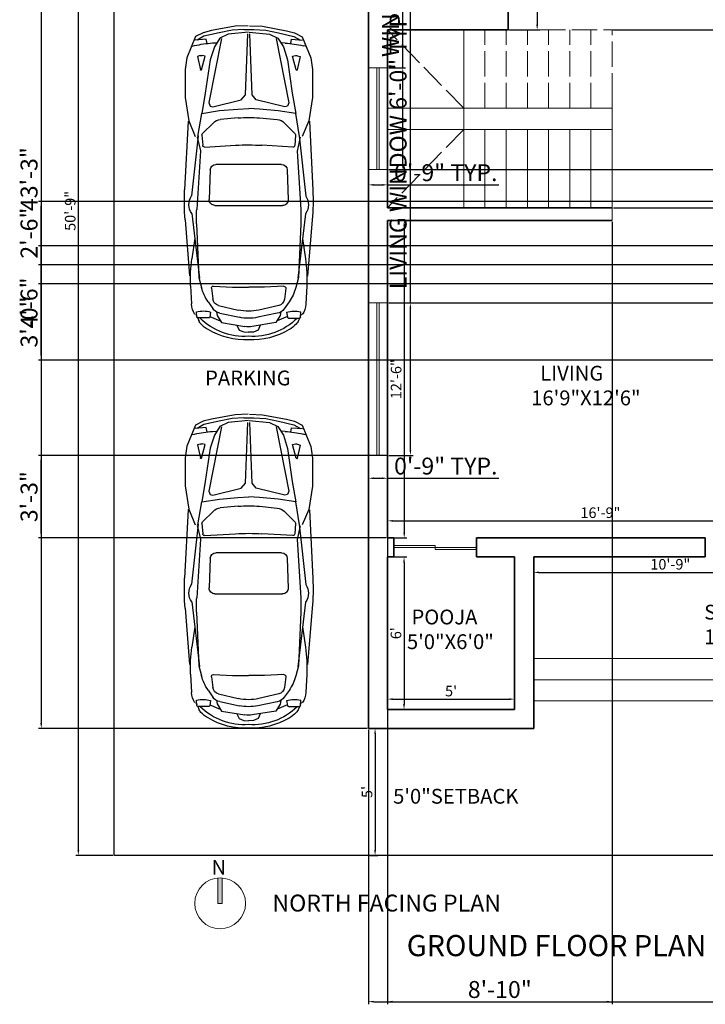
# Model space of a CAD drawing. Units: inches. Extents: x 3394 to 4794, y 965 to 1718.
# Tile 12 of 15: x 4177 to 4500, y 987 to 1453. Entities that reach past the tile are written whole.
import ezdxf

# ---------------------------------------------------------------- set-up
doc = ezdxf.new("R2010")
doc.units = ezdxf.units.IN
doc.linetypes.add('ACAD_ISO02W100', pattern=[15, 12, -3])
for name, color, linetype, lineweight in [('A-ANNO-DIMS', 2, 'Continuous', 13), ('A-ANNO-SYMB', 7, 'Continuous', 18), ('A-ANNO-TEXT', 7, 'Continuous', 18), ('A-ANNO-TITL', 7, 'Continuous', 25), ('A-AREA-IDEN', 7, 'Continuous', 18), ('A-DOOR', 4, 'Continuous', 18), ('A-FLOR-STRS', 7, 'Continuous', 18), ('A-FLOR-STRS-OVHD', 7, 'ACAD_ISO02W100', 13), ('A-GLAZ', 4, 'Continuous', 18), ('A-WALL', 7, 'Continuous', 35), ('C-PRKG-VEHI', 8, 'Continuous', 13), ('C-PROP', 7, 'Continuous', 25)]:
    doc.layers.add(name, color=color, linetype=linetype, lineweight=lineweight)
doc.layers.add('L9012X$0', color=2, linetype='Continuous')
doc.styles.get("Standard").update_dxf_attribs({"font": 'arial.ttf'})
doc.dimstyles.new('ISO-25', dxfattribs={"dimtxt": 8, "dimasz": 2.5, "dimexe": 1.25, "dimexo": 0.625, "dimtad": 1, "dimlunit": 3, "dimtxsty": 'Standard', "dimcen": 2.5, "dimadec": 0, "dimazin": 0, "dimtfac": 1, "dimtmove": 0, "dimatfit": 3, "dimfxl": 1, "dimarcsym": 0})

# ---------------------------------------------------------------- blocks, each defined once
blk = doc.blocks.new('A1099DC')
at = {"color": 0, "linetype": 'ByBlock'}
for p, q in [((1279.298465, 804.448389), (2201.430588, 851.890505)), ((2602.736326, 846.078152), (3356.693814, 785.353187)), ((139.051458, 595.027331), (190.951238, 683.213377)), ((179.200345, 564.515703), (190.951238, 709.631982)), ((272.228253, 749.073842), (265.114727, 718.465169)), ((398.733388, 644.315148), (411.280494, 678.748261)), ((411.280494, 678.748261), (588.616917, 641.417897)), ((1482.852352, 674.283145), (1175.286956, 622.180789)), ((1475.52921, 670.226262), (2282.402739, 758.004075)), ((1494.603245, 682.841284), (1678.210958, 641.166865)), ((1678.210958, 641.166865), (2462.684993, 690.847736)), ((2519.280414, 756.817792), (3387.476361, 653.818028)), ((2656.476214, 692.831247), (3376.704709, 662.004075)), ((2851.341839, 715.213377), (3126.60716, 755.701993)), ((3376.704709, 662.004075), (3510.708679, 626.736433)), ((3488.458929, 772.663345), (3732.658862, 759.86454)), ((3909.27561, 688.812956), (3837.725727, 693.401722)), ((3867.794139, 700.329656), (3900.059395, 686.767505)), ((3921.162781, 527.618662), (3921.162781, 676.138994)), ((3925.383812, 676.122818), (3955.306409, 663.545364)), ((92.537504, 388.14361), (139.051458, 595.027331)), ((236.043912, 551.980927), (179.200345, 564.515703)), ((405.405047, 577.538958), (396.874865, 615.894428)), ((589.014326, 626.599587), (405.405047, 577.538958)), ((1300.814287, 466.658131), (1445.712032, 613.104998)), ((1465.665584, 620.56924), (1602.893878, 610.287296)), ((1626.354615, 583.507504), (1602.652901, 169.222264)), ((3704.596898, 536.993674), (3795.675135, 473.385795)), ((229.117398, 477.634662), (225.714299, 427.957563)), ((1860.238743, -448.635916), (1859.369151, 433.397797)), ((1933.148906, 509.557888), (2330.980062, 522.200075)), ((2409.60024, 445.938054), (2410.49349, -460.09121)), ((3493.960271, 465.734554), (3507.923021, 209.166865)), ((3522.252709, 492.345257), (3666.066199, 475.644444)), ((3753.293176, 397.789551), (3815.226005, 132.124765)), ((3839.396146, 426.841284), (3888.358202, 417.538958)), ((3841.786866, 503.451367), (3910.58243, 515.096797)), ((3888.358202, 417.538958), (3983.199613, 359.957848)), ((3901.001848, 514.780764), (3957.150905, 375.772812)), ((57.774444, 216.608726), (92.537504, 388.14361)), ((1235.045743, 136.116317), (1257.419842, 373.755108)), ((3857.610793, 379.525702), (3912.067615, 118.157673)), ((3983.199613, 359.957848), (4035.448301, 43.94997)), ((49.168662, 58.00681), (57.774444, 216.608726)), ((3507.923021, 209.166865), (3507.64153, -4.333678)), ((4019.086894, 150.376168), (4084.69605, 122.469191)), ((4084.69605, 122.469191), (4109.177079, 60.329656)), ((4109.177079, 60.329656), (4113.094043, -5.158716)), ((49.301278, -76.507426), (58.219773, -235.092064)), ((3508.347273, -221.154823), (3507.644805, -7.65525)), ((3858.370276, -390.823819), (3912.311631, -129.348921)), ((3983.920268, -371.008369), (4035.545755, -54.898082)), ((4084.948231, -133.320044), (4109.306686, -71.132359)), ((4109.306686, -71.132359), (4113.094514, -5.636391)), ((58.219773, -235.092064), (93.320996, -406.558069)), ((1235.330373, -152.586046), (1258.173002, -390.180259)), ((1627.520644, -599.204785), (1603.002095, -184.967086)), ((3494.890446, -477.749545), (3508.347273, -221.154823)), ((3754.088875, -409.293325), (3815.497749, -143.506937)), ((4019.394229, -161.356334), (4084.948231, -133.320044)), ((3889.19258, -428.776374), (3983.920268, -371.008369)), ((3902.027941, -525.993061), (3957.902795, -386.874665)), ((93.320996, -406.558069), (140.24279, -613.349673)), ((230.077082, -495.779641), (226.576036, -446.109349)), ((1301.750547, -482.997536), (1446.936772, -629.158411)), ((1934.168526, -524.650381), (2332.023837, -536.508105)), ((3523.2353, -504.304409), (3667.01558, -487.320059)), ((3705.667171, -548.593196), (3796.61981, -484.805853)), ((3840.248961, -438.175225), (3889.19258, -428.776374)), ((3842.790735, -514.780444), (3911.609128, -526.290202)), ((140.24279, -613.349673), (192.316354, -701.433212)), ((237.150178, -570.112104), (180.331436, -582.758939)), ((180.331436, -582.758939), (192.368445, -727.851766)), ((406.561378, -595.336142), (398.106841, -633.708356)), ((590.267037, -644.034637), (406.561378, -595.336142)), ((412.636377, -696.533662), (589.898847, -658.853701)), ((1484.19765, -690.263206), (1176.530118, -638.767405)), ((1466.905004, -636.583294), (1604.112757, -626.030785)), ((1495.965396, -698.798158), (1679.490579, -656.761786)), ((1679.490579, -656.761786), (2464.061049, -704.895745)), ((3378.022114, -674.249887), (3511.956283, -638.718087)), ((3922.214148, -538.79118), (3922.506998, -687.311224)), ((273.723073, -767.133288), (266.549207, -736.538701)), ((400.0214, -662.125356), (412.636377, -696.533662)), ((1476.866524, -686.22077), (2283.911563, -772.40743)), ((2520.786439, -770.754078), (3388.777604, -666.042617)), ((2657.855804, -706.497136), (3378.022114, -674.249887)), ((2852.765183, -728.494989), (3128.109803, -768.440762)), ((3489.994314, -784.688586), (3734.168535, -771.408296)), ((3910.644841, -700.0086), (3839.104145, -704.738438)), ((3869.186159, -711.60707), (3901.424611, -697.981326)), ((3926.727989, -687.286725), (3956.625729, -674.650294)), ((1280.900818, -820.829563), (2203.124693, -866.453338)), ((2604.418191, -859.849707), (3358.254477, -797.638217))]:
    blk.add_line(p, q, dxfattribs=at)
for points in [[(-0.000783, 0.794772), (5.385043, 172.701749), (63.649891, 493.818028), (92.537504, 603.957563), (144.437284, 705.166865), (428.417214, 824.236633), (585.095796, 846.190121), (961.406447, 846.190121), (1274.27399, 797.818028), (1482.852352, 709.631982)], [(83.345007, -3.206171), (111.32237, 268.957533), (164.563706, 379.583828), (279.999271, 453.709838), (456.549665, 511.628518), (901.254996, 574.918954), (1175.286956, 622.180789), (1137.52997, 385.548359), (1118.345181, 137.317882), (1109.829198, -8.358455)], [(168.178729, 359.003083), (1030.214866, 528.397865), (1077.798844, 510.531569), (1086.170082, 475.285426), (992.832238, 91.960378), (924.218938, 35.478085), (108.447994, 6.034416)], [(0.019119, -19.392451), (5.743899, -191.288474), (64.641806, -512.289243), (93.746535, -622.371603), (145.845778, -723.478374), (430.059935, -841.987962), (586.7815, -863.632471), (963.091723, -863.198028), (1275.863278, -814.209121), (1484.26735, -725.611974)], [(83.356858, -15.227176), (111.870816, -287.335185), (165.330179, -397.856284), (280.911681, -471.754535), (457.575935, -529.324983), (902.4055, -592.045995), (1176.530118, -638.767405), (1138.306616, -402.209884), (1118.632407, -154.017717), (1109.829198, -8.358455)], [(168.904615, -377.268451), (1031.273389, -545.270714), (1078.822046, -527.310627), (1087.123771, -492.048047), (993.030273, -108.907787), (924.305735, -52.560894), (108.478017, -24.418246)]]:
    blk.add_lwpolyline(points, dxfattribs=at)
for centre, radius, start, end in [((2358.037832, -2192.08357), 3048, 85.395244, 92.945173), ((2399.99649, 588.663508), 206.166238, 54.649181, 124.776949), ((1749.553982, 373.478072), 1524, 166.916578, 176.08111), ((2578.271641, -1134.295865), 1828.8, 87.549126, 93.623712), ((3392.740754, -1053.630025), 1828.8, 86.999806, 98.367602), ((3718.678317, 475.802507), 284.405862, 57.329946, 87.182375), ((4191.049821, 605.937201), 363.988953, 166.096081, 196.353514), ((3908.462781, 676.138994), 12.7, 0, 86.330429), ((3896.252417, 523.051998), 152.4, 46.38363, 67.20138), ((446.46332, 626.922805), 50.8, 159.97873, 192.538409), ((587.047263, 633.961317), 7.62, 284.960009, 78.112462), ((1463.767788, 595.240237), 25.4, 85.715073, 135.304647), ((1600.996082, 584.958293), 25.4, 356.725615, 85.715073), ((3355.555414, 37.211519), 609.6, 55.070043, 75.255062), ((3320.85101, 50.338397), 847.430844, 356.245089, 44.519453), ((3700.933354, 318.064082), 435.542335, 30.457681, 46.38363), ((3204.184594, 25.950693), 1011.814461, 358.069446, 30.457681), ((1409.148822, 359.469565), 152.4, 135.304647, 174.62136), ((1935.569151, 433.396333), 76.2, 91.82012, 179.9989), ((2333.400307, 446.03852), 76.2, 359.924458, 91.82012), ((3519.322741, 467.114813), 25.4, 83.37601, 183.115039), ((3654.346327, 374.722669), 101.6, 13.122645, 83.37601), ((3708.414764, 348.440256), 152.4, 11.769371, 55.070043), ((3908.462781, 527.618662), 12.7, 279.607718, 0), ((2752.335538, -6.739118), 1524, 174.62136, 185.491615), ((4645.676894, -4.872483), 3048, 176.725615, 183.38736), ((1266.577845, -8.050136), 1219.2, 176.894161, 183.218814), ((3221.54491, -6.276527), 609.6, 346.99033, 13.122645), ((3315.283499, -6.18411), 609.6, 348.343604, 11.769371), ((3734.73098, -5.770579), 304.8, 350.724636, 9.388339), ((3320.962449, -62.69553), 847.430844, 315.593523, 3.867886), ((3204.248172, -38.537915), 1011.814461, 329.655294, 2.043529), ((1409.873518, -375.595566), 152.4, 185.491615, 224.808328), ((3709.113243, -360.032616), 152.4, 305.042932, 348.343604), ((1750.305335, -388.625277), 1524, 184.031865, 193.196397), ((1936.438592, -448.484202), 76.2, 180.114076, 268.292856), ((2334.293902, -460.341926), 76.2, 268.292856, 0.188517), ((3520.255588, -479.079792), 25.4, 176.997936, 276.736965), ((3655.096735, -386.42159), 101.6, 276.736965, 346.99033), ((4192.255091, -616.577407), 363.988953, 163.759461, 194.016894), ((3909.514173, -538.816222), 12.7, 0.112975, 80.505257), ((447.716945, -644.638934), 50.8, 167.574566, 200.134245), ((588.314493, -651.400231), 7.62, 282.000513, 75.152966), ((1464.957267, -611.258083), 25.4, 224.808328, 274.397903), ((1602.165021, -600.705574), 25.4, 274.397903, 3.38736), ((3355.640902, -49.500248), 609.6, 284.857913, 305.042932), ((3897.294828, -534.273643), 152.4, 292.911596, 313.729345), ((3701.571953, -329.671253), 435.542335, 313.729345, 329.655294), ((2401.171182, -602.835323), 206.166238, 235.336026, 305.463794), ((2576.048678, 1120.472221), 1828.8, 266.489263, 272.563849), ((3390.675263, 1041.412497), 1828.8, 261.745373, 273.113169), ((3719.627907, -487.374382), 284.405862, 272.930601, 302.78303), ((3909.807023, -687.336265), 12.7, 273.782546, 0.112975), ((2353.729565, 2177.823616), 3048, 267.167802, 274.717731)]:
    blk.add_arc(centre, radius, start, end, dxfattribs=at)
blk = doc.blocks.new('VI')
at = {"layer": 'L9012X$0'}
blk.add_blockref('A1099DC', (0, 0), dxfattribs=at)
blk = doc.blocks.new('*D33')
at = {"layer": 'A-ANNO-DIMS', "color": 0, "lineweight": -2, "transparency": 16777216}
for p, q in [((4407.9, 1573.68), (4422.16, 1573.68)), ((4420.91, 1571.18), (4420.91, 1450.18)), ((4407.9, 1447.68), (4422.16, 1447.68))]:
    blk.add_line(p, q, dxfattribs=at)
at = {"layer": 'A-ANNO-DIMS', "color": 0, "transparency": 16777216}
for points in [[(4420.49, 1571.18), (4421.33, 1571.18), (4420.91, 1573.68)], [(4420.49, 1450.18), (4421.33, 1450.18), (4420.91, 1447.68)]]:
    blk.add_solid(points, dxfattribs=at)
at = {"layer": 'Defpoints', "color": 0, "transparency": 16777216}
for p in [(4407.27, 1573.68), (4407.27, 1447.68), (4420.91, 1447.68)]:
    blk.add_point(p, dxfattribs=at)
at = {"layer": 'A-ANNO-DIMS', "color": 0, "transparency": 16777216, "insert": (4417.73, 1510.68), "char_height": 5, "attachment_point": 5, "rotation": 90}
blk.add_mtext('10\'-6"', dxfattribs=at)
blk = doc.blocks.new('*D34')
at = {"layer": 'A-ANNO-DIMS', "color": 0, "lineweight": -2, "transparency": 16777216}
for p, q in [((4350.9, 1198.68), (4359.32, 1198.68)), ((4358.07, 1196.18), (4358.07, 1129.18)), ((4350.9, 1126.68), (4359.32, 1126.68))]:
    blk.add_line(p, q, dxfattribs=at)
at = {"layer": 'A-ANNO-DIMS', "color": 0, "transparency": 16777216}
for points in [[(4357.65, 1196.18), (4358.48, 1196.18), (4358.07, 1198.68)], [(4357.65, 1129.18), (4358.48, 1129.18), (4358.07, 1126.68)]]:
    blk.add_solid(points, dxfattribs=at)
at = {"layer": 'Defpoints', "color": 0, "transparency": 16777216}
for p in [(4350.27, 1198.68), (4350.27, 1126.68), (4358.07, 1126.68)]:
    blk.add_point(p, dxfattribs=at)
at = {"layer": 'A-ANNO-DIMS', "color": 0, "transparency": 16777216, "insert": (4354.89, 1162.68), "char_height": 5, "attachment_point": 5, "rotation": 90}
blk.add_mtext("6'", dxfattribs=at)
blk = doc.blocks.new('*D35')
at = {"layer": 'A-ANNO-DIMS', "color": 0, "lineweight": -2, "transparency": 16777216}
for p, q in [((4350.27, 1127.31), (4350.27, 1132.77)), ((4352.77, 1131.52), (4407.77, 1131.52)), ((4410.27, 1127.31), (4410.27, 1132.77))]:
    blk.add_line(p, q, dxfattribs=at)
at = {"layer": 'A-ANNO-DIMS', "color": 0, "transparency": 16777216}
for points in [[(4352.77, 1131.94), (4352.77, 1131.11), (4350.27, 1131.52)], [(4407.77, 1131.94), (4407.77, 1131.11), (4410.27, 1131.52)]]:
    blk.add_solid(points, dxfattribs=at)
at = {"layer": 'Defpoints', "color": 0, "transparency": 16777216}
for p in [(4410.27, 1131.52), (4350.27, 1126.68), (4410.27, 1126.68)]:
    blk.add_point(p, dxfattribs=at)
at = {"layer": 'A-ANNO-DIMS', "color": 0, "transparency": 16777216, "insert": (4380.27, 1134.69), "char_height": 5, "attachment_point": 5}
blk.add_mtext("5'", dxfattribs=at)
blk = doc.blocks.new('*D36')
at = {"layer": 'A-ANNO-DIMS', "color": 0, "lineweight": -2, "transparency": 16777216}
for p, q in [((4419.27, 1198.06), (4419.27, 1190.15)), ((4548.27, 1198.06), (4548.27, 1190.15)), ((4421.77, 1191.4), (4545.77, 1191.4))]:
    blk.add_line(p, q, dxfattribs=at)
at = {"layer": 'A-ANNO-DIMS', "color": 0, "transparency": 16777216}
for points in [[(4421.77, 1191.81), (4421.77, 1190.98), (4419.27, 1191.4)], [(4545.77, 1191.81), (4545.77, 1190.98), (4548.27, 1191.4)]]:
    blk.add_solid(points, dxfattribs=at)
at = {"layer": 'Defpoints', "color": 0, "transparency": 16777216}
for p in [(4419.27, 1198.68), (4548.27, 1198.68), (4548.27, 1191.4)]:
    blk.add_point(p, dxfattribs=at)
at = {"layer": 'A-ANNO-DIMS', "color": 0, "transparency": 16777216, "insert": (4483.77, 1194.58), "char_height": 5, "attachment_point": 5}
blk.add_mtext('10\'-9"', dxfattribs=at)
blk = doc.blocks.new('*D39')
at = {"layer": 'A-ANNO-DIMS', "color": 0, "lineweight": -2, "transparency": 16777216}
for p, q in [((4341.9, 1117.68), (4345.65, 1117.68)), ((4344.4, 1115.18), (4344.4, 1060.18)), ((4341.9, 1057.68), (4345.65, 1057.68))]:
    blk.add_line(p, q, dxfattribs=at)
at = {"layer": 'A-ANNO-DIMS', "color": 0, "transparency": 16777216}
for points in [[(4343.99, 1115.18), (4344.82, 1115.18), (4344.4, 1117.68)], [(4343.99, 1060.18), (4344.82, 1060.18), (4344.4, 1057.68)]]:
    blk.add_solid(points, dxfattribs=at)
at = {"layer": 'Defpoints', "color": 0, "transparency": 16777216}
for p in [(4341.27, 1117.68), (4341.27, 1057.68), (4344.4, 1057.68)]:
    blk.add_point(p, dxfattribs=at)
at = {"layer": 'A-ANNO-DIMS', "color": 0, "transparency": 16777216, "insert": (4341.24, 1087.68), "char_height": 5, "attachment_point": 5, "rotation": 90}
blk.add_mtext("5'", dxfattribs=at)
blk = doc.blocks.new('*D40')
at = {"layer": 'A-ANNO-DIMS', "color": 0, "lineweight": -2, "transparency": 16777216}
for p, q in [((4350.9, 1357.68), (4359.41, 1357.68)), ((4358.16, 1355.18), (4358.16, 1210.18)), ((4350.9, 1207.68), (4359.41, 1207.68))]:
    blk.add_line(p, q, dxfattribs=at)
at = {"layer": 'A-ANNO-DIMS', "color": 0, "transparency": 16777216}
for points in [[(4357.74, 1355.18), (4358.57, 1355.18), (4358.16, 1357.68)], [(4357.74, 1210.18), (4358.57, 1210.18), (4358.16, 1207.68)]]:
    blk.add_solid(points, dxfattribs=at)
at = {"layer": 'Defpoints', "color": 0, "transparency": 16777216}
for p in [(4350.27, 1357.68), (4350.27, 1207.68), (4358.16, 1207.68)]:
    blk.add_point(p, dxfattribs=at)
at = {"layer": 'A-ANNO-DIMS', "color": 0, "transparency": 16777216, "insert": (4354.98, 1282.68), "char_height": 5, "attachment_point": 5, "rotation": 90}
blk.add_mtext('12\'-6"', dxfattribs=at)
blk = doc.blocks.new('*D41')
at = {"layer": 'A-ANNO-DIMS', "color": 0, "lineweight": -2, "transparency": 16777216}
for p, q in [((4350.27, 1208.31), (4350.27, 1217.01)), ((4352.77, 1215.76), (4548.77, 1215.76)), ((4551.27, 1208.31), (4551.27, 1217.01))]:
    blk.add_line(p, q, dxfattribs=at)
at = {"layer": 'A-ANNO-DIMS', "color": 0, "transparency": 16777216}
for points in [[(4352.77, 1216.17), (4352.77, 1215.34), (4350.27, 1215.76)], [(4548.77, 1216.17), (4548.77, 1215.34), (4551.27, 1215.76)]]:
    blk.add_solid(points, dxfattribs=at)
at = {"layer": 'Defpoints', "color": 0, "transparency": 16777216}
for p in [(4551.27, 1215.76), (4350.27, 1207.68), (4551.27, 1207.68)]:
    blk.add_point(p, dxfattribs=at)
at = {"layer": 'A-ANNO-DIMS', "color": 0, "transparency": 16777216, "insert": (4450.77, 1218.94), "char_height": 5, "attachment_point": 5}
blk.add_mtext('16\'-9"', dxfattribs=at)
blk = doc.blocks.new('*D53')
at = {"layer": 'A-ANNO-DIMS', "color": 0, "lineweight": -2, "transparency": 16777216}
for p, q in [((4220.65, 1666.68), (4203.08, 1666.68)), ((4204.33, 1060.18), (4204.33, 1664.18)), ((4220.65, 1057.68), (4203.08, 1057.68))]:
    blk.add_line(p, q, dxfattribs=at)
at = {"layer": 'A-ANNO-DIMS', "color": 0, "transparency": 16777216}
for points in [[(4203.92, 1664.18), (4204.75, 1664.18), (4204.33, 1666.68)], [(4203.92, 1060.18), (4204.75, 1060.18), (4204.33, 1057.68)]]:
    blk.add_solid(points, dxfattribs=at)
at = {"layer": 'Defpoints', "color": 0, "transparency": 16777216}
for p in [(4204.33, 1666.68), (4221.27, 1666.68), (4221.27, 1057.68)]:
    blk.add_point(p, dxfattribs=at)
at = {"layer": 'A-ANNO-DIMS', "color": 0, "transparency": 16777216, "insert": (4201.15, 1362.18), "char_height": 5, "attachment_point": 5, "rotation": 90}
blk.add_mtext('50\'-9"', dxfattribs=at)
blk = doc.blocks.new('WIN-48IN')
for p, q in [((9, 48), (0, 48)), ((4, 0), (4, 48)), ((5, 0), (5, 48)), ((9, 0), (0, 0))]:
    blk.add_line(p, q)
blk = doc.blocks.new('WIN-72IN')
for p, q in [((9, 72), (0, 72)), ((4, 0), (4, 72)), ((5, 0), (5, 72)), ((9, 0), (0, 0))]:
    blk.add_line(p, q)
blk = doc.blocks.new('DOOR-SLIDING-39IN')
for p, q in [((0, 2), (19.5, 2)), ((0, 1), (39, 1)), ((19.5, 2), (19.5, 0)), ((19.5, 0), (39, 0))]:
    blk.add_line(p, q)
blk = doc.blocks.new('NORTH-ARROW-PLAN')
at = {"transparency": 33554687}
h = blk.add_hatch(color=256, dxfattribs=at)
h.dxf.hatch_style = 1
h.paths.add_polyline_path([(13, 12), (11, 12), (11, 23.96, -0.020861), (12, 24, -0.020861), (13, 23.96)])
for p, q in [((11, 24), (11, 12)), ((13, 12), (13, 23.96)), ((11, 12), (13, 12))]:
    blk.add_line(p, q)
blk.add_circle((12, 12), 12)
blk.add_text('N', height=6.9).set_placement((7.98, 25.6))
blk = doc.blocks.new('STAIR-SITOUT-3STEP')
for p, q in [((129, 68), (129, 20)), ((139, 68), (139, 10)), ((149, 68), (149, 0)), ((0, 20), (129, 20)), ((0, 10), (139, 10)), ((0, 0), (149, 0))]:
    blk.add_line(p, q)
blk = doc.blocks.new('*D62')
at = {"layer": 'A-ANNO-DIMS', "color": 0, "lineweight": -2, "transparency": 16777216}
for p, q in [((4357.47, 1429.68), (4357.47, 1534.67)), ((4350.9, 1429.68), (4358.72, 1429.68)), ((4357.47, 1384.18), (4357.47, 1427.18)), ((4350.9, 1381.68), (4358.72, 1381.68))]:
    blk.add_line(p, q, dxfattribs=at)
at = {"layer": 'A-ANNO-DIMS', "color": 0, "transparency": 16777216}
for points in [[(4357.05, 1427.18), (4357.89, 1427.18), (4357.47, 1429.68)], [(4357.05, 1384.18), (4357.89, 1384.18), (4357.47, 1381.68)]]:
    blk.add_solid(points, dxfattribs=at)
at = {"layer": 'Defpoints', "color": 0, "transparency": 16777216}
for p in [(4350.27, 1429.68), (4357.47, 1429.68), (4350.27, 1381.68)]:
    blk.add_point(p, dxfattribs=at)
at = {"layer": 'A-ANNO-DIMS', "color": 0, "transparency": 16777216, "insert": (4352.71, 1483.42), "char_height": 8, "attachment_point": 5, "rotation": 90}
blk.add_mtext('WINDOW 4\'-0" TYP.', dxfattribs=at)
blk = doc.blocks.new('*D63')
at = {"layer": 'A-ANNO-DIMS', "color": 0, "lineweight": -2, "transparency": 16777216}
for p, q in [((4341.27, 1381.06), (4341.27, 1373.23)), ((4350.27, 1381.06), (4350.27, 1373.23)), ((4343.77, 1374.48), (4347.77, 1374.48)), ((4350.27, 1374.48), (4402.78, 1374.48))]:
    blk.add_line(p, q, dxfattribs=at)
at = {"layer": 'A-ANNO-DIMS', "color": 0, "transparency": 16777216}
for points in [[(4343.77, 1374.9), (4343.77, 1374.07), (4341.27, 1374.48)], [(4347.77, 1374.9), (4347.77, 1374.07), (4350.27, 1374.48)]]:
    blk.add_solid(points, dxfattribs=at)
at = {"layer": 'Defpoints', "color": 0, "transparency": 16777216}
for p in [(4341.27, 1381.68), (4350.27, 1381.68), (4350.27, 1374.48)]:
    blk.add_point(p, dxfattribs=at)
at = {"layer": 'A-ANNO-DIMS', "color": 0, "transparency": 16777216, "insert": (4377.78, 1379.19), "char_height": 8, "attachment_point": 5}
blk.add_mtext('0\'-9" TYP.', dxfattribs=at)
blk = doc.blocks.new('*D66')
at = {"layer": 'A-ANNO-DIMS', "color": 0, "lineweight": -2, "transparency": 16777216}
for p, q in [((4361.07, 1318.68), (4361.07, 1462.73)), ((4350.9, 1318.68), (4362.32, 1318.68)), ((4361.07, 1249.18), (4361.07, 1316.18)), ((4350.9, 1246.68), (4362.32, 1246.68))]:
    blk.add_line(p, q, dxfattribs=at)
at = {"layer": 'A-ANNO-DIMS', "color": 0, "transparency": 16777216}
for points in [[(4360.65, 1316.18), (4361.49, 1316.18), (4361.07, 1318.68)], [(4360.65, 1249.18), (4361.49, 1249.18), (4361.07, 1246.68)]]:
    blk.add_solid(points, dxfattribs=at)
at = {"layer": 'Defpoints', "color": 0, "transparency": 16777216}
for p in [(4350.27, 1318.68), (4361.07, 1318.68), (4350.27, 1246.68)]:
    blk.add_point(p, dxfattribs=at)
at = {"layer": 'A-ANNO-DIMS', "color": 0, "transparency": 16777216, "insert": (4356.31, 1391.96), "char_height": 8, "attachment_point": 5, "rotation": 90}
blk.add_mtext('LIVING WINDOW 6\'-0" TYP.', dxfattribs=at)
blk = doc.blocks.new('*D67')
at = {"layer": 'A-ANNO-DIMS', "color": 0, "lineweight": -2, "transparency": 16777216}
for p, q in [((4341.27, 1246.06), (4341.27, 1234.63)), ((4350.27, 1246.06), (4350.27, 1234.63)), ((4343.77, 1235.88), (4347.77, 1235.88)), ((4350.27, 1235.88), (4402.78, 1235.88))]:
    blk.add_line(p, q, dxfattribs=at)
at = {"layer": 'A-ANNO-DIMS', "color": 0, "transparency": 16777216}
for points in [[(4343.77, 1236.3), (4343.77, 1235.47), (4341.27, 1235.88)], [(4347.77, 1236.3), (4347.77, 1235.47), (4350.27, 1235.88)]]:
    blk.add_solid(points, dxfattribs=at)
at = {"layer": 'Defpoints', "color": 0, "transparency": 16777216}
for p in [(4341.27, 1246.68), (4350.27, 1246.68), (4350.27, 1235.88)]:
    blk.add_point(p, dxfattribs=at)
at = {"layer": 'A-ANNO-DIMS', "color": 0, "transparency": 16777216, "insert": (4377.78, 1240.59), "char_height": 8, "attachment_point": 5}
blk.add_mtext('0\'-9" TYP.', dxfattribs=at)
blk = doc.blocks.new('*D106')
at = {"layer": 'A-ANNO-DIMS', "color": 0, "lineweight": -2, "transparency": 16777216}
for p, q in [((4704.27, 1198.06), (4704.27, 987.36)), ((4341.27, 1117.06), (4341.27, 987.36)), ((4343.77, 988.61), (4701.77, 988.61))]:
    blk.add_line(p, q, dxfattribs=at)
at = {"layer": 'A-ANNO-DIMS', "color": 0, "transparency": 16777216}
for points in [[(4343.77, 989.03), (4343.77, 988.2), (4341.27, 988.61)], [(4701.77, 989.03), (4701.77, 988.2), (4704.27, 988.61)]]:
    blk.add_solid(points, dxfattribs=at)
at = {"layer": 'Defpoints', "color": 0, "transparency": 16777216}
for p in [(4704.27, 1198.68), (4341.27, 1117.68), (4704.27, 988.61)]:
    blk.add_point(p, dxfattribs=at)
at = {"layer": 'A-ANNO-DIMS', "color": 0, "transparency": 16777216, "insert": (4522.77, 993.32), "char_height": 8, "attachment_point": 5}
blk.add_mtext('30\'-3"', dxfattribs=at)
blk = doc.blocks.new('*D107')
at = {"layer": 'A-ANNO-DIMS', "color": 0, "lineweight": -2, "transparency": 16777216}
for p, q in [((4397.65, 1636.68), (4185.57, 1636.68)), ((4186.82, 1634.18), (4186.82, 1120.18)), ((4340.65, 1117.68), (4185.57, 1117.68))]:
    blk.add_line(p, q, dxfattribs=at)
at = {"layer": 'A-ANNO-DIMS', "color": 0, "transparency": 16777216}
for points in [[(4186.4, 1634.18), (4187.24, 1634.18), (4186.82, 1636.68)], [(4186.4, 1120.18), (4187.24, 1120.18), (4186.82, 1117.68)]]:
    blk.add_solid(points, dxfattribs=at)
at = {"layer": 'Defpoints', "color": 0, "transparency": 16777216}
for p in [(4398.27, 1636.68), (4186.82, 1117.68), (4341.27, 1117.68)]:
    blk.add_point(p, dxfattribs=at)
at = {"layer": 'A-ANNO-DIMS', "color": 0, "transparency": 16777216, "insert": (4182.11, 1377.18), "char_height": 8, "attachment_point": 5, "rotation": 90}
blk.add_mtext('43\'-3"', dxfattribs=at)
blk = doc.blocks.new('*D108')
at = {"layer": 'A-ANNO-DIMS', "color": 0, "lineweight": -2, "transparency": 16777216}
for p, q in [((4350.27, 1357.06), (4350.27, 987.36)), ((4456.27, 1357.06), (4456.27, 987.36)), ((4352.77, 988.61), (4453.77, 988.61))]:
    blk.add_line(p, q, dxfattribs=at)
at = {"layer": 'A-ANNO-DIMS', "color": 0, "transparency": 16777216}
for points in [[(4352.77, 989.03), (4352.77, 988.2), (4350.27, 988.61)], [(4453.77, 989.03), (4453.77, 988.2), (4456.27, 988.61)]]:
    blk.add_solid(points, dxfattribs=at)
at = {"layer": 'Defpoints', "color": 0, "transparency": 16777216}
for p in [(4350.27, 1357.68), (4456.27, 1357.68), (4456.27, 988.61)]:
    blk.add_point(p, dxfattribs=at)
at = {"layer": 'A-ANNO-DIMS', "color": 0, "transparency": 16777216, "insert": (4403.27, 993.32), "char_height": 8, "attachment_point": 5}
blk.add_mtext('8\'-10"', dxfattribs=at)
blk = doc.blocks.new('*D109')
at = {"layer": 'A-ANNO-DIMS', "color": 0, "lineweight": -2, "transparency": 16777216}
for p, q in [((4456.9, 1447.68), (4769.97, 1447.68)), ((4768.72, 1366.18), (4768.72, 1445.18)), ((4456.9, 1363.68), (4769.97, 1363.68))]:
    blk.add_line(p, q, dxfattribs=at)
at = {"layer": 'A-ANNO-DIMS', "color": 0, "transparency": 16777216}
for points in [[(4768.3, 1445.18), (4769.14, 1445.18), (4768.72, 1447.68)], [(4768.3, 1366.18), (4769.14, 1366.18), (4768.72, 1363.68)]]:
    blk.add_solid(points, dxfattribs=at)
at = {"layer": 'Defpoints', "color": 0, "transparency": 16777216}
for p in [(4456.27, 1447.68), (4768.72, 1447.68), (4456.27, 1363.68)]:
    blk.add_point(p, dxfattribs=at)
at = {"layer": 'A-ANNO-DIMS', "color": 0, "transparency": 16777216, "insert": (4764.01, 1405.68), "char_height": 8, "attachment_point": 5, "rotation": 90}
blk.add_mtext('7\'-0"', dxfattribs=at)
blk = doc.blocks.new('*D112')
at = {"layer": 'A-ANNO-DIMS', "color": 0, "lineweight": -2, "transparency": 16777216}
for p, q in [((4559.65, 1327.68), (4185.57, 1327.68)), ((4186.82, 1294.18), (4186.82, 1325.18)), ((4559.41, 1291.68), (4185.57, 1291.68))]:
    blk.add_line(p, q, dxfattribs=at)
at = {"layer": 'A-ANNO-DIMS', "color": 0, "transparency": 16777216}
for points in [[(4186.4, 1325.18), (4187.24, 1325.18), (4186.82, 1327.68)], [(4186.4, 1294.18), (4187.24, 1294.18), (4186.82, 1291.68)]]:
    blk.add_solid(points, dxfattribs=at)
at = {"layer": 'Defpoints', "color": 0, "transparency": 16777216}
for p in [(4186.82, 1327.68), (4560.27, 1327.68), (4560.03, 1291.68)]:
    blk.add_point(p, dxfattribs=at)
at = {"layer": 'A-ANNO-DIMS', "color": 0, "transparency": 16777216, "insert": (4182.11, 1309.68), "char_height": 8, "attachment_point": 5, "rotation": 90}
blk.add_mtext('3\'-0"', dxfattribs=at)
blk = doc.blocks.new('*D113')
at = {"layer": 'A-ANNO-DIMS', "color": 0, "lineweight": -2, "transparency": 16777216}
for p, q in [((4604.65, 1366.68), (4185.57, 1366.68)), ((4186.82, 1339.18), (4186.82, 1364.18)), ((4604.65, 1336.68), (4185.57, 1336.68))]:
    blk.add_line(p, q, dxfattribs=at)
at = {"layer": 'A-ANNO-DIMS', "color": 0, "transparency": 16777216}
for points in [[(4186.4, 1364.18), (4187.24, 1364.18), (4186.82, 1366.68)], [(4186.4, 1339.18), (4187.24, 1339.18), (4186.82, 1336.68)]]:
    blk.add_solid(points, dxfattribs=at)
at = {"layer": 'Defpoints', "color": 0, "transparency": 16777216}
for p in [(4186.82, 1366.68), (4605.27, 1366.68), (4605.27, 1336.68)]:
    blk.add_point(p, dxfattribs=at)
at = {"layer": 'A-ANNO-DIMS', "color": 0, "transparency": 16777216, "insert": (4182.11, 1351.68), "char_height": 8, "attachment_point": 5, "rotation": 90}
blk.add_mtext('2\'-6"', dxfattribs=at)
blk = doc.blocks.new('*D115')
at = {"layer": 'A-ANNO-DIMS', "color": 0, "lineweight": -2, "transparency": 16777216}
for p, q in [((4349.65, 1246.68), (4185.57, 1246.68)), ((4186.82, 1210.18), (4186.82, 1244.18)), ((4349.65, 1207.68), (4185.57, 1207.68))]:
    blk.add_line(p, q, dxfattribs=at)
at = {"layer": 'A-ANNO-DIMS', "color": 0, "transparency": 16777216}
for points in [[(4186.4, 1244.18), (4187.24, 1244.18), (4186.82, 1246.68)], [(4186.4, 1210.18), (4187.24, 1210.18), (4186.82, 1207.68)]]:
    blk.add_solid(points, dxfattribs=at)
at = {"layer": 'Defpoints', "color": 0, "transparency": 16777216}
for p in [(4186.82, 1246.68), (4350.27, 1246.68), (4350.27, 1207.68)]:
    blk.add_point(p, dxfattribs=at)
at = {"layer": 'A-ANNO-DIMS', "color": 0, "transparency": 16777216, "insert": (4182.11, 1227.18), "char_height": 8, "attachment_point": 5, "rotation": 90}
blk.add_mtext('3\'-3"', dxfattribs=at)
blk = doc.blocks.new('*D116')
at = {"layer": 'A-ANNO-DIMS', "color": 0, "lineweight": -2, "transparency": 16777216}
for p, q in [((4350.9, 1381.68), (4769.97, 1381.68)), ((4768.72, 1321.18), (4768.72, 1379.18)), ((4350.9, 1318.68), (4769.97, 1318.68))]:
    blk.add_line(p, q, dxfattribs=at)
at = {"layer": 'A-ANNO-DIMS', "color": 0, "transparency": 16777216}
for points in [[(4768.3, 1379.18), (4769.14, 1379.18), (4768.72, 1381.68)], [(4768.3, 1321.18), (4769.14, 1321.18), (4768.72, 1318.68)]]:
    blk.add_solid(points, dxfattribs=at)
at = {"layer": 'Defpoints', "color": 0, "transparency": 16777216}
for p in [(4350.27, 1381.68), (4768.72, 1381.68), (4350.27, 1318.68)]:
    blk.add_point(p, dxfattribs=at)
at = {"layer": 'A-ANNO-DIMS', "color": 0, "transparency": 16777216, "insert": (4764.01, 1350.18), "char_height": 8, "attachment_point": 5, "rotation": 90}
blk.add_mtext('5\'-3"', dxfattribs=at)
blk = doc.blocks.new('*D119')
at = {"layer": 'A-ANNO-DIMS', "color": 0, "lineweight": -2, "transparency": 16777216}
for p, q in [((4694.65, 1345.68), (4185.57, 1345.68)), ((4186.82, 1294.18), (4186.82, 1343.18)), ((4694.65, 1291.68), (4185.57, 1291.68))]:
    blk.add_line(p, q, dxfattribs=at)
at = {"layer": 'A-ANNO-DIMS', "color": 0, "transparency": 16777216}
for points in [[(4186.4, 1343.18), (4187.24, 1343.18), (4186.82, 1345.68)], [(4186.4, 1294.18), (4187.24, 1294.18), (4186.82, 1291.68)]]:
    blk.add_solid(points, dxfattribs=at)
at = {"layer": 'Defpoints', "color": 0, "transparency": 16777216}
for p in [(4186.82, 1345.68), (4695.27, 1345.68), (4695.27, 1291.68)]:
    blk.add_point(p, dxfattribs=at)
at = {"layer": 'A-ANNO-DIMS', "color": 0, "transparency": 16777216, "insert": (4182.11, 1318.68), "char_height": 8, "attachment_point": 5, "rotation": 90}
blk.add_mtext('4\'-6"', dxfattribs=at)

msp = doc.modelspace()

# ---------------------------------------------------------------- linework, layer by layer
at = {"layer": 'A-FLOR-STRS'}
for p, q in [((4386.27, 1363.682), (4386.27, 1447.682)), ((4456.27, 1357.682), (4456.27, 1415.182)), ((4350.27, 1410.682), (4456.27, 1410.682)), ((4350.27, 1400.682), (4456.27, 1400.682)), ((4396.27, 1363.682), (4396.27, 1400.682)), ((4406.27, 1363.682), (4406.27, 1400.682)), ((4416.27, 1363.682), (4416.27, 1400.682)), ((4426.27, 1363.682), (4426.27, 1400.682)), ((4436.27, 1363.682), (4436.27, 1400.682)), ((4446.27, 1363.682), (4446.27, 1400.682))]:
    msp.add_line(p, q, dxfattribs=at)
at = {"layer": 'A-FLOR-STRS-OVHD'}
for p, q in [((4386.27, 1410.682), (4350.27, 1447.682)), ((4396.27, 1410.682), (4396.27, 1447.682)), ((4406.27, 1410.682), (4406.27, 1447.682)), ((4407.27, 1447.682), (4457.27, 1447.682)), ((4416.27, 1410.682), (4416.27, 1447.682)), ((4426.27, 1410.682), (4426.27, 1447.682)), ((4436.27, 1410.682), (4436.27, 1447.682)), ((4446.27, 1410.682), (4446.27, 1447.682)), ((4456.27, 1415.182), (4456.27, 1447.682)), ((4386.27, 1400.682), (4350.27, 1363.682))]:
    msp.add_line(p, q, dxfattribs=at)
at = {"layer": 'A-WALL'}
for p, q in [((4407.27, 1573.682), (4407.27, 1447.682)), ((4341.27, 1117.682), (4341.27, 1456.682)), ((4350.27, 1447.682), (4407.27, 1447.682)), ((4350.27, 1363.682), (4350.27, 1447.682)), ((4350.27, 1363.682), (4456.27, 1363.682)), ((4350.27, 1357.682), (4456.27, 1357.682)), ((4350.27, 1207.682), (4350.27, 1357.682)), ((4350.27, 1207.682), (4353.27, 1207.682)), ((4353.27, 1198.682), (4353.27, 1207.682)), ((4392.27, 1207.682), (4500.27, 1207.682)), ((4392.27, 1198.682), (4392.27, 1207.682)), ((4500.27, 1207.682), (4500.27, 1198.682)), ((4350.27, 1198.682), (4353.27, 1198.682)), ((4350.27, 1126.682), (4350.27, 1198.682)), ((4392.27, 1198.682), (4410.27, 1198.682)), ((4410.27, 1126.682), (4410.27, 1198.682)), ((4419.27, 1198.682), (4500.27, 1198.682)), ((4419.27, 1117.682), (4419.27, 1198.682)), ((4410.27, 1126.682), (4350.27, 1126.682)), ((4419.27, 1117.682), (4341.27, 1117.682))]:
    msp.add_line(p, q, dxfattribs=at)
at = {"layer": 'C-PROP'}
for p, q in [((4221.27, 1057.682), (4221.27, 1666.682)), ((4734.27, 1057.682), (4221.27, 1057.682))]:
    msp.add_line(p, q, dxfattribs=at)

# ---------------------------------------------------------------- block references
at = {"layer": 'A-ANNO-SYMB'}
msp.add_blockref('NORTH-ARROW-PLAN', (4259.247, 1023.062), dxfattribs=at)
at = {"layer": 'A-DOOR'}
msp.add_blockref('DOOR-SLIDING-39IN', (4353.271, 1202.182), dxfattribs=at)
at = {"layer": 'A-FLOR-STRS'}
msp.add_blockref('STAIR-SITOUT-3STEP', (4419.271, 1130.682), dxfattribs=at)
at = {"layer": 'A-GLAZ'}
for name, p in [('WIN-48IN', (4341.271, 1381.682)), ('WIN-72IN', (4341.271, 1246.682))]:
    msp.add_blockref(name, p, dxfattribs=at)
at = {"layer": 'C-PRKG-VEHI', "xscale": -0.0351896714874634, "yscale": 0.0351896714874634, "zscale": 0.0351896714874634, "rotation": 90}
for p in [(4284.498, 1449.569), (4284.498, 1266.085)]:
    msp.add_blockref('VI', p, dxfattribs=at)

# ---------------------------------------------------------------- texts
at = {"layer": 'A-ANNO-TEXT', "insert": (4352.914, 1089.143), "char_height": 7, "attachment_point": 1}
msp.add_mtext_dynamic_manual_height_columns('{\\fTimes New Roman|b0|i0|c0|p18;5\'0"SETBACK}', width=61.05572, gutter_width=12.5, heights=[0], dxfattribs=at)
at = {"layer": 'A-ANNO-TITL', "attachment_point": 1}
for s, insert, char_height in [('{\\fTimes New Roman|b0|i0|c0|p18;NORTH FACING PLAN}', (4295.94, 1039.185), 8), ('{\\fTimes New Roman|b0|i0|c0|p18;GROUND FLOOR PLAN}', (4359.341, 1020.098), 10)]:
    msp.add_mtext_dynamic_manual_height_columns(s, width=196.26071, gutter_width=12.5, heights=[0], dxfattribs=dict(at, insert=insert, char_height=char_height))
at = {"layer": 'A-AREA-IDEN', "char_height": 7, "attachment_point": 1}
for s, insert in [('{\\fTimes New Roman|b0|i0|c0|p18;  LIVING\\P16\'9"X12\'6"}', (4418.088, 1289)), ('{\\fTimes New Roman|b0|i0|c0|p18;PARKING}', (4264.15, 1286.731)), ('{\\fTimes New Roman|b0|i0|c0|p18; POOJA\\P5\'0"X6\'0"}', (4359.438, 1173.83)), ('{\\fTimes New Roman|b0|i0|c0|p18;SITOUT\\P10\'6"X4\'0"}', (4499.74, 1176.113))]:
    msp.add_mtext_dynamic_manual_height_columns(s, width=61.05572, gutter_width=12.5, heights=[0], dxfattribs=dict(at, insert=insert))

# ---------------------------------------------------------------- dimensions: what is measured, and where the dimension line sits
at = {"layer": 'A-ANNO-DIMS'}
for base, p1, p2, override, picture, middle in [((4204.332, 1666.682), (4221.27, 1057.682), (4221.27, 1666.682), {"dimtxt": 5, "dimclrd": 0, "dimclre": 0, "dimclrt": 0}, '*D53', (4201.154, 1362.182)), ((4186.82, 1117.682), (4398.27, 1636.682), (4341.27, 1117.682), {"dimdec": 1, "dimlfac": 1, "dimrnd": 0, "dimzin": 1, "dimdsep": 46, "dimlunit": 4, "dimfrac": 2}, '*D107', (4182.108, 1377.182)), ((4420.911, 1447.682), (4407.27, 1573.682), (4407.27, 1447.682), {"dimtxt": 5, "dimclrd": 0, "dimclre": 0, "dimclrt": 0}, '*D33', (4417.733, 1510.682)), ((4768.72, 1447.682), (4456.27, 1363.682), (4456.27, 1447.682), {"dimdec": 1, "dimlfac": 1, "dimrnd": 0, "dimzin": 1, "dimdsep": 46, "dimlunit": 4, "dimfrac": 2}, '*D109', (4764.011, 1405.682)), ((4768.72, 1381.682), (4350.27, 1318.682), (4350.27, 1381.682), {"dimdec": 1, "dimlfac": 1, "dimrnd": 0, "dimzin": 1, "dimdsep": 46, "dimlunit": 4, "dimfrac": 2}, '*D116', (4764.008, 1350.182)), ((4186.82, 1366.682), (4605.27, 1336.682), (4605.27, 1366.682), {"dimdec": 1, "dimlfac": 1, "dimrnd": 0, "dimzin": 1, "dimdsep": 46, "dimlunit": 4, "dimfrac": 2}, '*D113', (4182.111, 1351.682)), ((4358.156, 1207.682), (4350.27, 1357.682), (4350.27, 1207.682), {"dimtxt": 5, "dimclrd": 0, "dimclre": 0, "dimclrt": 0}, '*D40', (4354.978, 1282.682)), ((4186.82, 1345.682), (4695.27, 1291.682), (4695.27, 1345.682), {"dimdec": 1, "dimlfac": 1, "dimrnd": 0, "dimzin": 1, "dimdsep": 46, "dimlunit": 4, "dimfrac": 2}, '*D119', (4182.111, 1318.682)), ((4186.82, 1327.682), (4560.035, 1291.683), (4560.27, 1327.682), {"dimdec": 1, "dimlfac": 1, "dimrnd": 0, "dimzin": 1, "dimdsep": 46, "dimlunit": 4, "dimfrac": 2}, '*D112', (4182.108, 1309.683)), ((4186.82, 1246.682), (4350.27, 1207.682), (4350.27, 1246.682), {"dimdec": 1, "dimlfac": 1, "dimrnd": 0, "dimzin": 1, "dimdsep": 46, "dimlunit": 4, "dimfrac": 2}, '*D115', (4182.108, 1227.182)), ((4358.067, 1126.682), (4350.27, 1198.682), (4350.27, 1126.682), {"dimtxt": 5, "dimclrd": 0, "dimclre": 0, "dimclrt": 0}, '*D34', (4354.889, 1162.682)), ((4344.403, 1057.682), (4341.27, 1117.682), (4341.27, 1057.682), {"dimtxt": 5, "dimclrd": 0, "dimclre": 0, "dimclrt": 0}, '*D39', (4341.236, 1087.682))]:
    dim = msp.add_linear_dim(base=base, p1=p1, p2=p2, angle=90, dimstyle='ISO-25', override=override, dxfattribs=at)
    dim.commit()
    dim.dimension.update_dxf_attribs({"geometry": picture, "text_midpoint": middle})
for base, p1, p2, text, picture, middle in [((4357.47, 1429.682), (4350.27, 1381.682), (4350.27, 1429.682), 'WINDOW <> TYP.', '*D62', (4352.706, 1483.424)), ((4361.07, 1318.682), (4350.27, 1246.682), (4350.27, 1318.682), 'LIVING WINDOW <> TYP.', '*D66', (4356.306, 1391.957))]:
    dim = msp.add_linear_dim(base=base, p1=p1, p2=p2, angle=90, text=text, dimstyle='ISO-25', override={"dimdec": 1, "dimlfac": 1, "dimrnd": 0, "dimzin": 1, "dimdsep": 46, "dimlunit": 4, "dimfrac": 2}, dxfattribs=at)
    dim.commit()
    dim.dimension.update_dxf_attribs({"geometry": picture, "text_midpoint": middle})
for base, p1, p2, picture, middle in [((4350.27, 1374.482), (4341.27, 1381.682), (4350.27, 1381.682), '*D63', (4377.777, 1379.192)), ((4350.27, 1235.882), (4341.27, 1246.682), (4350.27, 1246.682), '*D67', (4377.777, 1240.592))]:
    dim = msp.add_linear_dim(base=base, p1=p1, p2=p2, text='<> TYP.', dimstyle='ISO-25', override={"dimdec": 1, "dimlfac": 1, "dimrnd": 0, "dimzin": 1, "dimdsep": 46, "dimlunit": 4, "dimfrac": 2}, dxfattribs=at)
    dim.commit()
    dim.dimension.update_dxf_attribs({"geometry": picture, "text_midpoint": middle})
for base, p1, p2, override, picture, middle in [((4456.27, 988.612), (4350.27, 1357.682), (4456.27, 1357.682), {"dimdec": 1, "dimlfac": 1, "dimrnd": 0, "dimzin": 1, "dimdsep": 46, "dimlunit": 4, "dimfrac": 2}, '*D108', (4403.27, 993.322)), ((4551.27, 1215.757), (4350.27, 1207.682), (4551.27, 1207.682), {"dimtxt": 5, "dimclrd": 0, "dimclre": 0, "dimclrt": 0}, '*D41', (4450.77, 1218.935)), ((4704.27, 988.612), (4341.27, 1117.682), (4704.27, 1198.682), {"dimdec": 1, "dimlfac": 1, "dimrnd": 0, "dimzin": 1, "dimdsep": 46, "dimlunit": 4, "dimfrac": 2}, '*D106', (4522.77, 993.325)), ((4548.27, 1191.398), (4419.27, 1198.682), (4548.27, 1198.682), {"dimtxt": 5, "dimclrd": 0, "dimclre": 0, "dimclrt": 0}, '*D36', (4483.77, 1194.575)), ((4410.27, 1131.522), (4350.27, 1126.682), (4410.27, 1126.682), {"dimtxt": 5, "dimclrd": 0, "dimclre": 0, "dimclrt": 0}, '*D35', (4380.27, 1134.69))]:
    dim = msp.add_linear_dim(base=base, p1=p1, p2=p2, dimstyle='ISO-25', override=override, dxfattribs=at)
    dim.commit()
    dim.dimension.update_dxf_attribs({"geometry": picture, "text_midpoint": middle})

doc.saveas('drawing.dxf')
